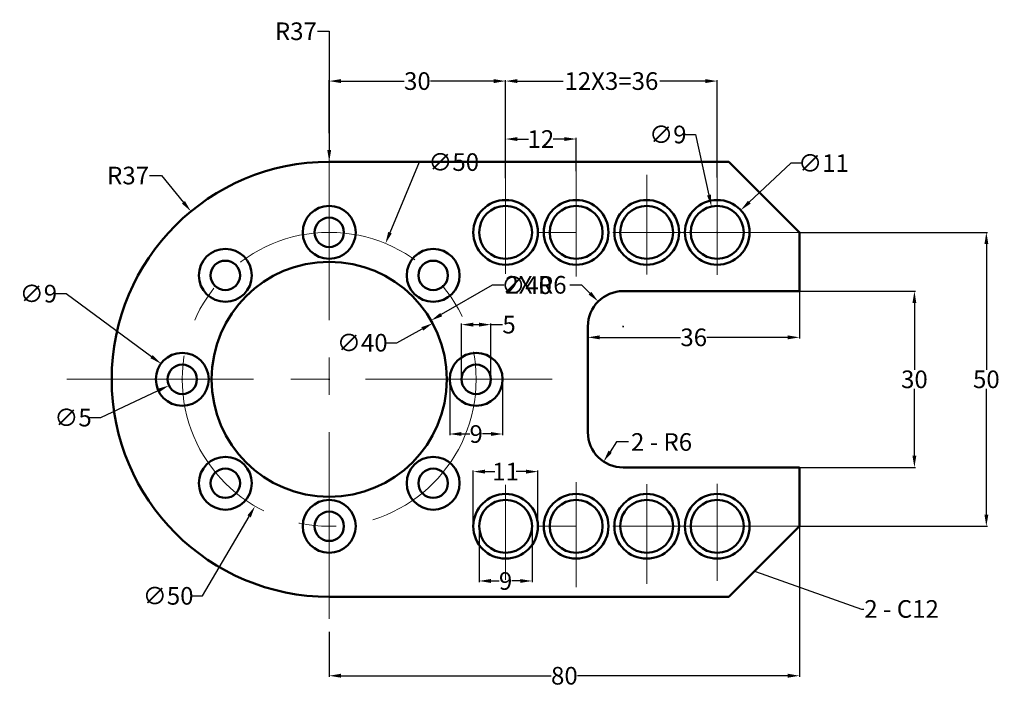
# Model space of a CAD drawing. Units: inches. Extents: x 142 to 309, y 90 to 204.
import ezdxf
from ezdxf import colors
from ezdxf.entities.mleader import LeaderData, LeaderLine
from ezdxf.math import Vec2, Vec3

# ---------------------------------------------------------------- set-up
doc = ezdxf.new("R2010")
doc.units = ezdxf.units.IN
doc.header["$MEASUREMENT"] = 0
doc.linetypes.add('CENTER', pattern=[50.8, 31.75, -6.35, 6.35, -6.35])
for name, color, linetype, lineweight in [('M-CNTR', 4, 'CENTER', 18), ('M-DIMS', 2, 'Continuous', 25), ('M-OUTL', 7, 'Continuous', 50)]:
    doc.layers.add(name, color=color, linetype=linetype, lineweight=lineweight)
doc.styles.get("Standard").update_dxf_attribs({"font": 'arial.ttf'})
doc.dimstyles.get("Standard").update_dxf_attribs({"dimtxt": 3, "dimasz": 2, "dimexe": 0.18, "dimexo": 0.0625, "dimgap": 0.09, "dimtad": 0, "dimtih": 1, "dimtoh": 1, "dimdec": 0, "dimzin": 0, "dimdsep": 46, "dimtxsty": 'Standard', "dimcen": 0.09, "dimclrd": 1, "dimclre": 1, "dimadec": 0, "dimazin": 0, "dimtfac": 1, "dimtdec": 0, "dimtofl": 0, "dimtmove": 0, "dimatfit": 3, "dimfxl": 1, "dimtolj": 1, "dimtzin": 0, "dimarcsym": 0})

# ---------------------------------------------------------------- blocks, each defined once
blk = doc.blocks.new('*U1')
for radius in [4.5, 2.5]:
    blk.add_circle((0, 0), radius)
blk = doc.blocks.new('*U2')
at = {"layer": 'M-OUTL', "color": 0, "linetype": 'ByBlock', "lineweight": -2, "transparency": 16777216}
blk.add_blockref('*U1', (77.26, 77.84), dxfattribs=at)
for p, rotation in [((59.59, 70.52), 45.00000000000001), ((94.94, 70.52), 315), ((52.26, 52.84), 90), ((102.26, 52.84), 270), ((59.59, 35.16), 135), ((94.94, 35.16), 225), ((77.26, 27.84), 180)]:
    blk.add_blockref('*U1', p, dxfattribs=dict(at, rotation=rotation))
blk = doc.blocks.new('*U3')
for radius in [5.5, 4.5]:
    blk.add_circle((0, 0), radius)
blk = doc.blocks.new('*U4')
at = {"layer": 'M-OUTL', "color": 0, "linetype": 'ByBlock', "lineweight": -2, "transparency": 16777216}
for p in [(224.47, 167.73), (236.47, 167.73), (248.47, 167.73), (260.47, 167.73)]:
    blk.add_blockref('*U3', p, dxfattribs=at)
blk = doc.blocks.new('*D5')
at = {"layer": 'Defpoints', "color": 0, "transparency": 16777216}
for p in [(224.47, 193.46), (194.47, 184.54), (224.47, 176.86)]:
    blk.add_point(p, dxfattribs=at)
at = {"layer": 'M-DIMS', "color": 0, "lineweight": -2, "transparency": 16777216}
for p, q in [((194.47, 184.61), (194.47, 193.64)), ((196.47, 193.46), (207.24, 193.46)), ((222.47, 193.46), (211.7, 193.46)), ((224.47, 176.93), (224.47, 193.64))]:
    blk.add_line(p, q, dxfattribs=at)
at = {"layer": 'M-DIMS', "color": 0, "transparency": 16777216}
for points in [[(196.47, 193.79), (196.47, 193.12), (194.47, 193.46)], [(222.47, 193.79), (222.47, 193.12), (224.47, 193.46)]]:
    blk.add_solid(points, dxfattribs=at)
at = {"layer": 'M-DIMS', "color": 0, "transparency": 16777216, "insert": (209.47, 193.46), "char_height": 3, "attachment_point": 5}
blk.add_mtext('\\A1;30', dxfattribs=at)
blk = doc.blocks.new('*D6')
at = {"layer": 'Defpoints', "color": 0, "transparency": 16777216}
for p in [(236.47, 183.6), (236.47, 178.06), (224.47, 176.86)]:
    blk.add_point(p, dxfattribs=at)
at = {"layer": 'M-DIMS', "color": 0, "lineweight": -2, "transparency": 16777216}
for p, q in [((224.47, 176.93), (224.47, 183.78)), ((226.47, 183.6), (228.39, 183.6)), ((234.47, 183.6), (232.55, 183.6)), ((236.47, 178.12), (236.47, 183.78))]:
    blk.add_line(p, q, dxfattribs=at)
at = {"layer": 'M-DIMS', "color": 0, "transparency": 16777216}
for points in [[(226.47, 183.93), (226.47, 183.27), (224.47, 183.6)], [(234.47, 183.93), (234.47, 183.27), (236.47, 183.6)]]:
    blk.add_solid(points, dxfattribs=at)
at = {"layer": 'M-DIMS', "color": 0, "transparency": 16777216, "insert": (230.47, 183.6), "char_height": 3, "attachment_point": 5}
blk.add_mtext('\\A1;12', dxfattribs=at)
blk = doc.blocks.new('*D7')
at = {"layer": 'Defpoints', "color": 0, "transparency": 16777216}
for p in [(260.47, 193.46), (224.47, 176.86), (260.47, 176.99)]:
    blk.add_point(p, dxfattribs=at)
at = {"layer": 'M-DIMS', "color": 0, "lineweight": -2, "transparency": 16777216}
for p, q in [((224.47, 176.93), (224.47, 193.64)), ((226.47, 193.46), (234.26, 193.46)), ((258.47, 193.46), (250.69, 193.46)), ((260.47, 177.05), (260.47, 193.64))]:
    blk.add_line(p, q, dxfattribs=at)
at = {"layer": 'M-DIMS', "color": 0, "transparency": 16777216}
for points in [[(226.47, 193.79), (226.47, 193.12), (224.47, 193.46)], [(258.47, 193.79), (258.47, 193.12), (260.47, 193.46)]]:
    blk.add_solid(points, dxfattribs=at)
at = {"layer": 'M-DIMS', "color": 0, "transparency": 16777216, "insert": (242.47, 193.46), "char_height": 3, "attachment_point": 5}
blk.add_mtext('\\A1;12X3=36', dxfattribs=at)
blk = doc.blocks.new('*D8')
at = {"layer": 'Defpoints', "color": 0, "transparency": 16777216}
for p in [(274.47, 157.73), (238.47, 149.87), (238.47, 149.87)]:
    blk.add_point(p, dxfattribs=at)
at = {"layer": 'M-DIMS', "color": 0, "lineweight": -2, "transparency": 16777216}
for p, q in [((274.47, 157.67), (274.47, 149.69)), ((238.47, 149.93), (238.47, 150.05)), ((240.47, 149.87), (254.23, 149.87)), ((272.47, 149.87), (258.71, 149.87))]:
    blk.add_line(p, q, dxfattribs=at)
at = {"layer": 'M-DIMS', "color": 0, "transparency": 16777216}
for points in [[(240.47, 150.2), (240.47, 149.53), (238.47, 149.87)], [(272.47, 150.2), (272.47, 149.53), (274.47, 149.87)]]:
    blk.add_solid(points, dxfattribs=at)
at = {"layer": 'M-DIMS', "color": 0, "transparency": 16777216, "insert": (256.47, 149.87), "char_height": 3, "attachment_point": 5}
blk.add_mtext('\\A1;36', dxfattribs=at)
blk = doc.blocks.new('*D9')
at = {"layer": 'Defpoints', "color": 0, "transparency": 16777216}
for p in [(244.47, 133.73), (241.14, 128.74)]:
    blk.add_point(p, dxfattribs=at)
at = {"layer": 'M-DIMS', "color": 0, "lineweight": -2, "transparency": 16777216}
for p, q in [((243.36, 132.07), (242.25, 130.4)), ((245.36, 132.07), (243.36, 132.07))]:
    blk.add_line(p, q, dxfattribs=at)
at = {"layer": 'M-DIMS', "color": 0, "transparency": 16777216}
blk.add_solid([(241.97, 130.59), (242.53, 130.22), (241.14, 128.74)], dxfattribs=at)
at = {"layer": 'M-DIMS', "color": 0, "transparency": 16777216, "insert": (251, 132.07), "char_height": 3, "attachment_point": 5}
blk.add_mtext('\\A1;2 - R6', dxfattribs=at)
blk = doc.blocks.new('*D10')
at = {"layer": 'Defpoints', "color": 0, "transparency": 16777216}
for p in [(170.95, 171.29), (194.47, 142.73)]:
    blk.add_point(p, dxfattribs=at)
at = {"layer": 'M-DIMS', "color": 0, "lineweight": -2, "transparency": 16777216}
for p, q in [((163.92, 177.39), (165.92, 177.39)), ((165.92, 177.39), (169.67, 172.83)), ((194.38, 142.73), (194.56, 142.73)), ((194.47, 142.64), (194.47, 142.82))]:
    blk.add_line(p, q, dxfattribs=at)
at = {"layer": 'M-DIMS', "color": 0, "transparency": 16777216}
blk.add_solid([(169.93, 173.04), (169.42, 172.62), (170.95, 171.29)], dxfattribs=at)
at = {"layer": 'M-DIMS', "color": 0, "transparency": 16777216, "insert": (160.25, 177.39), "char_height": 3, "attachment_point": 5}
blk.add_mtext('\\A1;R37', dxfattribs=at)
blk = doc.blocks.new('*D11')
at = {"layer": 'Defpoints', "color": 0, "transparency": 16777216}
for p in [(165.85, 145.4), (173.09, 140.06)]:
    blk.add_point(p, dxfattribs=at)
at = {"layer": 'M-DIMS', "color": 0, "lineweight": -2, "transparency": 16777216}
for p, q in [((147.71, 157.3), (149.71, 157.3)), ((149.71, 157.3), (164.24, 146.59)), ((169.38, 142.73), (169.56, 142.73)), ((169.47, 142.64), (169.47, 142.82))]:
    blk.add_line(p, q, dxfattribs=at)
at = {"layer": 'M-DIMS', "color": 0, "transparency": 16777216}
blk.add_solid([(164.44, 146.86), (164.04, 146.32), (165.85, 145.4)], dxfattribs=at)
at = {"layer": 'M-DIMS', "color": 0, "transparency": 16777216, "insert": (145, 157.3), "char_height": 3, "attachment_point": 5}
blk.add_mtext('\\A1;∅9', dxfattribs=at)
blk = doc.blocks.new('*D12')
at = {"layer": 'Defpoints', "color": 0, "transparency": 16777216}
for p in [(171.73, 143.79), (167.21, 141.67)]:
    blk.add_point(p, dxfattribs=at)
at = {"layer": 'M-DIMS', "color": 0, "lineweight": -2, "transparency": 16777216}
for p, q in [((169.38, 142.73), (169.56, 142.73)), ((169.47, 142.64), (169.47, 142.82)), ((155.61, 136.22), (165.4, 140.82)), ((153.61, 136.22), (155.61, 136.22))]:
    blk.add_line(p, q, dxfattribs=at)
at = {"layer": 'M-DIMS', "color": 0, "transparency": 16777216}
blk.add_solid([(165.26, 141.12), (165.54, 140.52), (167.21, 141.67)], dxfattribs=at)
at = {"layer": 'M-DIMS', "color": 0, "transparency": 16777216, "insert": (150.89, 136.22), "char_height": 3, "attachment_point": 5}
blk.add_mtext('\\A1;∅5', dxfattribs=at)
blk = doc.blocks.new('*D13')
at = {"layer": 'Defpoints', "color": 0, "transparency": 16777216}
for p in [(207.09, 164.31), (181.85, 121.15)]:
    blk.add_point(p, dxfattribs=at)
at = {"layer": 'M-DIMS', "color": 0, "lineweight": -2, "transparency": 16777216}
for p, q in [((194.38, 142.73), (194.56, 142.73)), ((194.47, 142.64), (194.47, 142.82)), ((172.94, 105.9), (180.84, 119.42)), ((170.94, 105.9), (172.94, 105.9))]:
    blk.add_line(p, q, dxfattribs=at)
at = {"layer": 'M-DIMS', "color": 0, "transparency": 16777216}
blk.add_solid([(180.56, 119.59), (181.13, 119.25), (181.85, 121.15)], dxfattribs=at)
at = {"layer": 'M-DIMS', "color": 0, "transparency": 16777216, "insert": (167.07, 105.9), "char_height": 3, "attachment_point": 5}
blk.add_mtext('\\A1;∅50', dxfattribs=at)
blk = doc.blocks.new('*D14')
at = {"layer": 'Defpoints', "color": 0, "transparency": 16777216}
for p in [(212.06, 152.26), (176.89, 133.2)]:
    blk.add_point(p, dxfattribs=at)
at = {"layer": 'M-DIMS', "color": 0, "lineweight": -2, "transparency": 16777216}
for p, q in [((205.96, 148.95), (210.3, 151.3)), ((203.96, 148.95), (205.96, 148.95))]:
    blk.add_line(p, q, dxfattribs=at)
at = {"layer": 'M-DIMS', "color": 0, "transparency": 16777216}
blk.add_solid([(210.14, 151.6), (210.46, 151.01), (212.06, 152.26)], dxfattribs=at)
at = {"layer": 'M-DIMS', "color": 0, "transparency": 16777216, "insert": (200.09, 148.95), "char_height": 3, "attachment_point": 5}
blk.add_mtext('\\A1;∅40', dxfattribs=at)
blk = doc.blocks.new('*D15')
at = {"layer": 'Defpoints', "color": 0, "transparency": 16777216}
for p in [(274.47, 157.73), (274.47, 127.73), (294.01, 127.73)]:
    blk.add_point(p, dxfattribs=at)
at = {"layer": 'M-DIMS', "color": 0, "lineweight": -2, "transparency": 16777216}
for p, q in [((274.53, 157.73), (294.19, 157.73)), ((294.01, 155.73), (294.01, 144.35)), ((294.01, 129.73), (294.01, 141.11)), ((274.53, 127.73), (294.19, 127.73))]:
    blk.add_line(p, q, dxfattribs=at)
at = {"layer": 'M-DIMS', "color": 0, "transparency": 16777216}
for points in [[(293.68, 155.73), (294.34, 155.73), (294.01, 157.73)], [(293.68, 129.73), (294.34, 129.73), (294.01, 127.73)]]:
    blk.add_solid(points, dxfattribs=at)
at = {"layer": 'M-DIMS', "color": 0, "transparency": 16777216, "insert": (294.01, 142.73), "char_height": 3, "attachment_point": 5}
blk.add_mtext('\\A1;30', dxfattribs=at)
blk = doc.blocks.new('*U16')
for radius in [5.5, 4.5]:
    blk.add_circle((0, 0), radius)
blk = doc.blocks.new('*U17')
at = {"layer": 'M-OUTL', "color": 0, "linetype": 'ByBlock', "lineweight": -2, "transparency": 16777216}
for p in [(224.47, 167.73), (236.47, 167.73), (248.47, 167.73), (260.47, 167.73)]:
    blk.add_blockref('*U16', p, dxfattribs=at)
blk = doc.blocks.new('*D18')
at = {"layer": 'Defpoints', "color": 0, "transparency": 16777216}
for p in [(274.47, 167.73), (274.47, 117.73), (306.25, 117.73)]:
    blk.add_point(p, dxfattribs=at)
at = {"layer": 'M-DIMS', "color": 0, "lineweight": -2, "transparency": 16777216}
for p, q in [((274.53, 167.73), (306.43, 167.73)), ((306.25, 165.73), (306.25, 144.35)), ((306.25, 119.73), (306.25, 141.11)), ((274.53, 117.73), (306.43, 117.73))]:
    blk.add_line(p, q, dxfattribs=at)
at = {"layer": 'M-DIMS', "color": 0, "transparency": 16777216}
for points in [[(305.92, 165.73), (306.59, 165.73), (306.25, 167.73)], [(305.92, 119.73), (306.59, 119.73), (306.25, 117.73)]]:
    blk.add_solid(points, dxfattribs=at)
at = {"layer": 'M-DIMS', "color": 0, "transparency": 16777216, "insert": (306.25, 142.73), "char_height": 3, "attachment_point": 5}
blk.add_mtext('\\A1;50', dxfattribs=at)
blk = doc.blocks.new('*D19')
at = {"layer": 'Defpoints', "color": 0, "transparency": 16777216}
for p in [(274.47, 117.73), (194.47, 99.83), (274.47, 92.31)]:
    blk.add_point(p, dxfattribs=at)
at = {"layer": 'M-DIMS', "color": 0, "lineweight": -2, "transparency": 16777216}
for p, q in [((274.47, 117.67), (274.47, 92.13)), ((194.47, 99.77), (194.47, 92.13)), ((196.47, 92.31), (232.24, 92.31)), ((272.47, 92.31), (236.71, 92.31))]:
    blk.add_line(p, q, dxfattribs=at)
at = {"layer": 'M-DIMS', "color": 0, "transparency": 16777216}
for points in [[(196.47, 92.65), (196.47, 91.98), (194.47, 92.31)], [(272.47, 92.65), (272.47, 91.98), (274.47, 92.31)]]:
    blk.add_solid(points, dxfattribs=at)
at = {"layer": 'M-DIMS', "color": 0, "transparency": 16777216, "insert": (234.47, 92.31), "char_height": 3, "attachment_point": 5}
blk.add_mtext('\\A1;80', dxfattribs=at)
blk = doc.blocks.new('*D20')
at = {"layer": 'Defpoints', "color": 0, "transparency": 16777216}
for p in [(264.48, 171.5), (256.47, 163.96)]:
    blk.add_point(p, dxfattribs=at)
at = {"layer": 'M-DIMS', "color": 0, "lineweight": -2, "transparency": 16777216}
for p, q in [((272.97, 179.5), (265.93, 172.87)), ((274.97, 179.5), (272.97, 179.5)), ((260.38, 167.73), (260.56, 167.73)), ((260.47, 167.64), (260.47, 167.82))]:
    blk.add_line(p, q, dxfattribs=at)
at = {"layer": 'M-DIMS', "color": 0, "transparency": 16777216}
blk.add_solid([(265.7, 173.11), (266.16, 172.63), (264.48, 171.5)], dxfattribs=at)
at = {"layer": 'M-DIMS', "color": 0, "transparency": 16777216, "insert": (278.55, 179.5), "char_height": 3, "attachment_point": 5}
blk.add_mtext('\\A1;∅11', dxfattribs=at)
blk = doc.blocks.new('*D21')
at = {"layer": 'Defpoints', "color": 0, "transparency": 16777216}
for p in [(259.5, 172.12), (261.45, 163.34)]:
    blk.add_point(p, dxfattribs=at)
at = {"layer": 'M-DIMS', "color": 0, "lineweight": -2, "transparency": 16777216}
for p, q in [((254.78, 184.37), (256.78, 184.37)), ((256.78, 184.37), (259.06, 174.08)), ((260.38, 167.73), (260.56, 167.73)), ((260.47, 167.64), (260.47, 167.82))]:
    blk.add_line(p, q, dxfattribs=at)
at = {"layer": 'M-DIMS', "color": 0, "transparency": 16777216}
blk.add_solid([(259.39, 174.15), (258.74, 174), (259.5, 172.12)], dxfattribs=at)
at = {"layer": 'M-DIMS', "color": 0, "transparency": 16777216, "insert": (252.07, 184.37), "char_height": 3, "attachment_point": 5}
blk.add_mtext('\\A1;∅9', dxfattribs=at)
blk = doc.blocks.new('*D22')
at = {"layer": 'Defpoints', "color": 0, "transparency": 16777216}
for p in [(221.97, 152.03), (216.97, 142.73), (221.97, 142.73)]:
    blk.add_point(p, dxfattribs=at)
at = {"layer": 'M-DIMS', "color": 1, "lineweight": -2, "transparency": 16777216}
for p, q in [((216.97, 142.79), (216.97, 152.21)), ((218.97, 152.03), (219.97, 152.03)), ((221.97, 142.79), (221.97, 152.21)), ((221.97, 152.03), (223.97, 152.03))]:
    blk.add_line(p, q, dxfattribs=at)
at = {"layer": 'M-DIMS', "color": 1, "transparency": 16777216}
for points in [[(218.97, 152.36), (218.97, 151.7), (216.97, 152.03)], [(219.97, 152.36), (219.97, 151.7), (221.97, 152.03)]]:
    blk.add_solid(points, dxfattribs=at)
at = {"layer": 'M-DIMS', "color": 0, "transparency": 16777216, "insert": (225.06, 152.03), "char_height": 3, "attachment_point": 5}
blk.add_mtext('\\A1;5', dxfattribs=at)
blk = doc.blocks.new('*D23')
at = {"layer": 'Defpoints', "color": 0, "transparency": 16777216}
for p in [(214.97, 142.73), (223.97, 142.73), (214.97, 133.43)]:
    blk.add_point(p, dxfattribs=at)
at = {"layer": 'M-DIMS', "color": 1, "lineweight": -2, "transparency": 16777216}
for p, q in [((214.97, 142.67), (214.97, 133.25)), ((223.97, 142.67), (223.97, 133.25)), ((216.97, 133.43), (218.39, 133.43)), ((221.97, 133.43), (220.55, 133.43))]:
    blk.add_line(p, q, dxfattribs=at)
at = {"layer": 'M-DIMS', "color": 1, "transparency": 16777216}
for points in [[(216.97, 133.76), (216.97, 133.1), (214.97, 133.43)], [(221.97, 133.76), (221.97, 133.1), (223.97, 133.43)]]:
    blk.add_solid(points, dxfattribs=at)
at = {"layer": 'M-DIMS', "color": 0, "transparency": 16777216, "insert": (219.47, 133.43), "char_height": 3, "attachment_point": 5}
blk.add_mtext('\\A1;9', dxfattribs=at)
blk = doc.blocks.new('*D24')
at = {"layer": 'Defpoints', "color": 0, "transparency": 16777216}
for p in [(219.97, 117.73), (228.97, 117.73), (219.97, 108.43)]:
    blk.add_point(p, dxfattribs=at)
at = {"layer": 'M-DIMS', "color": 1, "lineweight": -2, "transparency": 16777216}
for p, q in [((219.97, 117.67), (219.97, 108.25)), ((228.97, 117.67), (228.97, 108.25)), ((221.97, 108.43), (223.39, 108.43)), ((226.97, 108.43), (225.55, 108.43))]:
    blk.add_line(p, q, dxfattribs=at)
at = {"layer": 'M-DIMS', "color": 1, "transparency": 16777216}
for points in [[(221.97, 108.76), (221.97, 108.1), (219.97, 108.43)], [(226.97, 108.76), (226.97, 108.1), (228.97, 108.43)]]:
    blk.add_solid(points, dxfattribs=at)
at = {"layer": 'M-DIMS', "color": 0, "transparency": 16777216, "insert": (224.47, 108.43), "char_height": 3, "attachment_point": 5}
blk.add_mtext('\\A1;9', dxfattribs=at)
blk = doc.blocks.new('*D25')
at = {"layer": 'Defpoints', "color": 0, "transparency": 16777216}
for p in [(229.97, 127.03), (218.97, 117.73), (229.97, 117.73)]:
    blk.add_point(p, dxfattribs=at)
at = {"layer": 'M-DIMS', "color": 1, "lineweight": -2, "transparency": 16777216}
for p, q in [((218.97, 117.79), (218.97, 127.21)), ((220.97, 127.03), (222.66, 127.03)), ((227.97, 127.03), (226.28, 127.03)), ((229.97, 117.79), (229.97, 127.21))]:
    blk.add_line(p, q, dxfattribs=at)
at = {"layer": 'M-DIMS', "color": 1, "transparency": 16777216}
for points in [[(220.97, 127.36), (220.97, 126.7), (218.97, 127.03)], [(227.97, 127.36), (227.97, 126.7), (229.97, 127.03)]]:
    blk.add_solid(points, dxfattribs=at)
at = {"layer": 'M-DIMS', "color": 0, "transparency": 16777216, "insert": (224.47, 127.03), "char_height": 3, "attachment_point": 5}
blk.add_mtext('\\A1;11', dxfattribs=at)
blk = doc.blocks.new('*D26')
at = {"layer": 'Defpoints', "color": 0, "transparency": 16777216}
for p in [(194.47, 179.73), (194.47, 142.73)]:
    blk.add_point(p, dxfattribs=at)
at = {"layer": 'M-DIMS', "color": 1, "lineweight": -2, "transparency": 16777216}
for p, q in [((192.47, 201.93), (194.47, 201.93)), ((194.47, 201.93), (194.47, 181.73)), ((194.38, 142.73), (194.56, 142.73)), ((194.47, 142.64), (194.47, 142.82))]:
    blk.add_line(p, q, dxfattribs=at)
at = {"layer": 'M-DIMS', "color": 1, "transparency": 16777216}
blk.add_solid([(194.8, 181.73), (194.14, 181.73), (194.47, 179.73)], dxfattribs=at)
at = {"layer": 'M-DIMS', "color": 0, "transparency": 16777216, "insert": (188.8, 201.93), "char_height": 3, "attachment_point": 5}
blk.add_mtext('\\A1;R37', dxfattribs=at)
blk = doc.blocks.new('*D27')
at = {"layer": 'Defpoints', "color": 0, "transparency": 16777216}
for p in [(211.79, 152.73), (177.15, 132.73)]:
    blk.add_point(p, dxfattribs=at)
at = {"layer": 'M-DIMS', "color": 1, "lineweight": -2, "transparency": 16777216}
for p, q in [((222.18, 158.73), (213.52, 153.73)), ((224.18, 158.73), (222.18, 158.73)), ((194.38, 142.73), (194.56, 142.73)), ((194.47, 142.64), (194.47, 142.82))]:
    blk.add_line(p, q, dxfattribs=at)
at = {"layer": 'M-DIMS', "color": 1, "transparency": 16777216}
blk.add_solid([(213.36, 154.02), (213.69, 153.44), (211.79, 152.73)], dxfattribs=at)
at = {"layer": 'M-DIMS', "color": 0, "transparency": 16777216, "insert": (228.05, 158.73), "char_height": 3, "attachment_point": 5}
blk.add_mtext('\\A1;∅40', dxfattribs=at)
blk = doc.blocks.new('*D28')
at = {"layer": 'Defpoints', "color": 0, "transparency": 16777216}
for p in [(204.04, 165.83), (184.9, 119.63)]:
    blk.add_point(p, dxfattribs=at)
at = {"layer": 'M-DIMS', "color": 1, "lineweight": -2, "transparency": 16777216}
for p, q in [((209.78, 179.68), (204.8, 167.67)), ((211.78, 179.68), (209.78, 179.68)), ((194.38, 142.73), (194.56, 142.73)), ((194.47, 142.64), (194.47, 142.82))]:
    blk.add_line(p, q, dxfattribs=at)
at = {"layer": 'M-DIMS', "color": 1, "transparency": 16777216}
blk.add_solid([(204.5, 167.8), (205.11, 167.55), (204.04, 165.83)], dxfattribs=at)
at = {"layer": 'M-DIMS', "color": 0, "transparency": 16777216, "insert": (215.64, 179.68), "char_height": 3, "attachment_point": 5}
blk.add_mtext('\\A1;∅50', dxfattribs=at)
blk = doc.blocks.new('*D29')
at = {"layer": 'Defpoints', "color": 0, "transparency": 16777216}
for p in [(240.23, 155.97), (244.47, 151.73)]:
    blk.add_point(p, dxfattribs=at)
at = {"layer": 'M-DIMS', "color": 1, "lineweight": -2, "transparency": 16777216}
for p, q in [((235.4, 158.8), (237.4, 158.8)), ((237.4, 158.8), (238.81, 157.39)), ((244.38, 151.73), (244.56, 151.73)), ((244.47, 151.64), (244.47, 151.82))]:
    blk.add_line(p, q, dxfattribs=at)
at = {"layer": 'M-DIMS', "color": 1, "transparency": 16777216}
blk.add_solid([(239.05, 157.62), (238.58, 157.15), (240.23, 155.97)], dxfattribs=at)
at = {"layer": 'M-DIMS', "color": 0, "transparency": 16777216, "insert": (229.64, 158.8), "char_height": 3, "attachment_point": 5}
blk.add_mtext('\\A1;2X R6', dxfattribs=at)

msp = doc.modelspace()

# ---------------------------------------------------------------- linework, layer by layer
at = {"layer": 'M-CNTR'}
for p, q in [((194.47, 184.54), (194.47, 99.83)), ((236.47, 160.22), (236.47, 178.06)), ((224.47, 160.67), (224.47, 176.86)), ((248.47, 160.56), (248.47, 177.49)), ((260.47, 160.5), (260.47, 176.99)), ((274.47, 167.73), (224.47, 167.73)), ((149.82, 142.73), (238.47, 142.73)), ((224.47, 124.79), (224.47, 108.6)), ((236.47, 125.24), (236.47, 107.4)), ((248.47, 124.9), (248.47, 107.97)), ((260.47, 124.96), (260.47, 108.47)), ((274.47, 117.73), (224.47, 117.73))]:
    msp.add_line(p, q, dxfattribs=at)
msp.add_circle((194.47, 142.73), 25, dxfattribs=at)
at = {"layer": 'M-OUTL'}
for p, q in [((194.47, 179.73), (262.47, 179.73)), ((262.47, 179.73), (274.47, 167.73)), ((274.47, 157.73), (274.47, 167.73)), ((274.47, 167.73), (274.47, 167.73)), ((244.47, 157.73), (274.47, 157.73)), ((238.47, 133.73), (238.47, 151.73)), ((274.47, 127.73), (244.47, 127.73)), ((274.47, 127.73), (274.47, 117.73)), ((262.47, 105.73), (274.47, 117.73)), ((194.47, 105.73), (262.47, 105.73))]:
    msp.add_line(p, q, dxfattribs=at)
msp.add_circle((194.47, 142.73), 20, dxfattribs=at)
for centre, radius, start, end in [((194.47, 142.73), 37, 90, 270), ((244.47, 151.73), 6, 90, 180), ((244.47, 133.73), 6, 180, 270)]:
    msp.add_arc(centre, radius, start, end, dxfattribs=at)

# ---------------------------------------------------------------- block references
for name, p in [('*U4', (0, 0)), ('*U2', (117.21, 89.89))]:
    msp.add_blockref(name, p, dxfattribs=at)
at = {"layer": 'M-OUTL', "xscale": -1, "rotation": 180}
msp.add_blockref('*U17', (0, 285.46), dxfattribs=at)

# ---------------------------------------------------------------- dimensions: what is measured, and where the dimension line sits
at = {"layer": 'M-DIMS'}
for mpoint, override, picture, middle in [((194.47, 179.73), {"dimdec": 0, "dimlfac": 1, "dimrnd": 0, "dimzin": 0, "dimdsep": 46, "dimlunit": 2}, '*D26', (188.8, 201.93)), ((170.95, 171.29), {"dimclrd": 0, "dimclre": 0, "dimclrt": 0}, '*D10', (160.25, 177.39))]:
    dim = msp.add_radius_dim(center=(194.47, 142.73), mpoint=mpoint, dimstyle='Standard', override=override, dxfattribs=at)
    dim.commit()
    dim.dimension.update_dxf_attribs({"geometry": picture, "text_midpoint": middle, "dimtype": 164})
for base, p1, p2, override, picture, middle in [((224.47, 193.46), (194.47, 184.54), (224.47, 176.86), {"dimclrd": 0, "dimclre": 0, "dimclrt": 0}, '*D5', (209.47, 193.46)), ((236.47, 183.6), (224.47, 176.86), (236.47, 178.06), {"dimclrd": 0, "dimclre": 0, "dimclrt": 0}, '*D6', (230.47, 183.6)), ((221.97, 152.03), (216.97, 142.73), (221.97, 142.73), {"dimdec": 0, "dimlfac": 1, "dimrnd": 0, "dimzin": 0, "dimdsep": 46, "dimlunit": 2}, '*D22', (225.06, 152.03)), ((229.97, 127.03), (218.97, 117.73), (229.97, 117.73), {"dimdec": 0, "dimlfac": 1, "dimrnd": 0, "dimzin": 0, "dimdsep": 46, "dimlunit": 2}, '*D25', (224.47, 127.03)), ((274.47, 92.31), (194.47, 99.83), (274.47, 117.73), {"dimclrd": 0, "dimclre": 0, "dimclrt": 0}, '*D19', (234.47, 92.31))]:
    dim = msp.add_linear_dim(base=base, p1=p1, p2=p2, dimstyle='Standard', override=override, dxfattribs=at)
    dim.commit()
    dim.dimension.update_dxf_attribs({"geometry": picture, "text_midpoint": middle})
dim = msp.add_linear_dim(base=(260.47, 193.46), p1=(224.47, 176.86), p2=(260.47, 176.99), text='12X3=<>', dimstyle='Standard', override={"dimclrd": 0, "dimclre": 0, "dimclrt": 0}, dxfattribs=at)
dim.commit()
dim.dimension.update_dxf_attribs({"geometry": '*D7', "text_midpoint": (242.47, 193.46)})
for p1, p2, override, picture, middle in [((261.45, 163.34), (259.5, 172.12), {"dimclrd": 0, "dimclre": 0, "dimclrt": 0}, '*D21', (252.07, 184.37)), ((184.9, 119.63), (204.04, 165.83), {"dimdec": 0, "dimlfac": 1, "dimrnd": 0, "dimzin": 0, "dimdsep": 46, "dimlunit": 2}, '*D28', (215.64, 179.68)), ((256.47, 163.96), (264.48, 171.5), {"dimclrd": 0, "dimclre": 0, "dimclrt": 0}, '*D20', (278.55, 179.5)), ((207.09, 164.31), (181.85, 121.15), {"dimclrd": 0, "dimclre": 0, "dimclrt": 0}, '*D13', (167.07, 105.9)), ((173.09, 140.06), (165.85, 145.4), {"dimclrd": 0, "dimclre": 0, "dimclrt": 0}, '*D11', (145, 157.3)), ((177.15, 132.73), (211.79, 152.73), {"dimdec": 0, "dimlfac": 1, "dimrnd": 0, "dimzin": 0, "dimdsep": 46, "dimlunit": 2}, '*D27', (228.05, 158.73)), ((176.89, 133.2), (212.06, 152.26), {"dimclrd": 0, "dimclre": 0, "dimclrt": 0}, '*D14', (200.09, 148.95)), ((171.73, 143.79), (167.21, 141.67), {"dimclrd": 0, "dimclre": 0, "dimclrt": 0}, '*D12', (150.89, 136.22))]:
    dim = msp.add_diameter_dim_2p(p1=p1, p2=p2, dimstyle='Standard', override=override, dxfattribs=at)
    dim.commit()
    dim.dimension.update_dxf_attribs({"geometry": picture, "text_midpoint": middle, "dimtype": 163})
for base, p1, p2, angle, override, picture, middle in [((306.25, 117.73), (274.47, 167.73), (274.47, 117.73), 90, {"dimclrd": 0, "dimclre": 0, "dimclrt": 0}, '*D18', (306.25, 142.73)), ((238.47, 149.87), (274.47, 157.73), (238.47, 149.87), 180, {"dimclrd": 0, "dimclre": 0, "dimclrt": 0}, '*D8', (256.47, 149.87)), ((294.01, 127.73), (274.47, 157.73), (274.47, 127.73), 90, {"dimclrd": 0, "dimclre": 0, "dimclrt": 0}, '*D15', (294.01, 142.73)), ((214.97, 133.43), (223.97, 142.73), (214.97, 142.73), 180, {"dimdec": 0, "dimlfac": 1, "dimrnd": 0, "dimzin": 0, "dimdsep": 46, "dimlunit": 2}, '*D23', (219.47, 133.43)), ((219.97, 108.43), (228.97, 117.73), (219.97, 117.73), 180, {"dimdec": 0, "dimlfac": 1, "dimrnd": 0, "dimzin": 0, "dimdsep": 46, "dimlunit": 2}, '*D24', (224.47, 108.43))]:
    dim = msp.add_linear_dim(base=base, p1=p1, p2=p2, angle=angle, dimstyle='Standard', override=override, dxfattribs=at)
    dim.commit()
    dim.dimension.update_dxf_attribs({"geometry": picture, "text_midpoint": middle})
dim = msp.add_radius_dim(center=(244.47, 151.73), mpoint=(240.23, 155.97), text='2X <>', dimstyle='Standard', override={"dimdec": 0, "dimlfac": 1, "dimrnd": 0, "dimzin": 0, "dimdsep": 46, "dimlunit": 2}, dxfattribs=at)
dim.commit()
dim.dimension.update_dxf_attribs({"geometry": '*D29', "text_midpoint": (229.64, 158.8)})
dim = msp.add_radius_dim(center=(244.47, 133.73), mpoint=(241.14, 128.74), text='2 - <>', dimstyle='Standard', override={"dimclrd": 0, "dimclre": 0, "dimclrt": 0}, dxfattribs=at)
dim.commit()
dim.dimension.update_dxf_attribs({"geometry": '*D9', "text_midpoint": (251, 132.07), "dimtype": 164})

# ---------------------------------------------------------------- leaders
ml = msp.add_multileader_mtext('Standard', dxfattribs=at)
ml.set_content('2 - C12', color=256)
ml.set_leader_properties()
ml.build(insert=Vec2(0, 0))
ml.multileader.update_dxf_attribs({"dogleg_length": 0.36, "arrow_head_size": 0.18})
ctx = ml.context
ctx.base_point, ctx.char_height, ctx.arrow_head_size, ctx.landing_gap_size, ctx.plane_origin = Vec3(285.4, 103.64), 3, 0.18, 0.09, Vec3(266.83, 110.09)
notes = []
notes.append((ctx, [(0, (1, 1, 0), (285.04, 103.64), (1, 0), 0.36, [(0, [(266.83, 110.09)], 0, [])])]))
ctx.mtext.insert, ctx.mtext.width, ctx.mtext.flow_direction = Vec3(285.49, 105.17), 23.8108, 5
for ctx, leaders in notes:
    for number, flags, end, landing, length, lines in leaders:
        leader = LeaderData()
        leader.index, (leader.has_last_leader_line, leader.has_dogleg_vector, leader.attachment_direction) = number, flags
        leader.last_leader_point, leader.dogleg_vector, leader.dogleg_length = Vec3(end), Vec3(landing), length
        for number, points, colour, breaks in lines:
            line = LeaderLine()
            line.index, line.vertices, line.color, line.breaks = number, Vec3.list(points), colors.encode_raw_color(colour), breaks
            leader.lines.append(line)
        ctx.leaders.append(leader)

doc.saveas('drawing.dxf')
